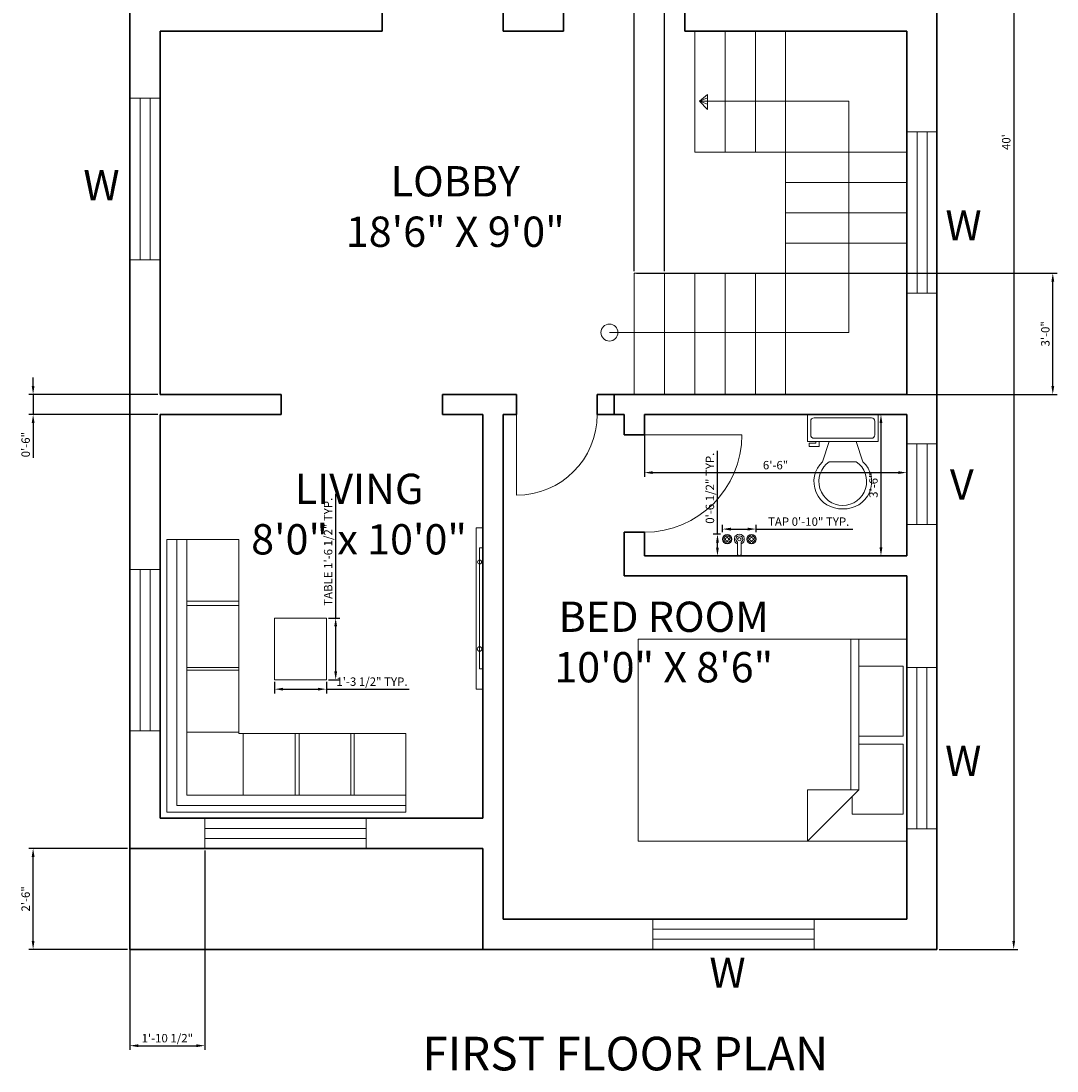
# Model space of a CAD drawing. Units: inches. Extents: x 1827 to 2455, y 1682 to 2281.
# Tile 2 of 3: x 2147 to 2455, y 1682 to 1994. Entities that reach past the tile are written whole.
import ezdxf

# ---------------------------------------------------------------- set-up
doc = ezdxf.new("R2010")
doc.units = ezdxf.units.IN
for name, color, linetype, lineweight in [('A-ANNO-DIMS', 2, 'Continuous', 18), ('A-ANNO-TEXT', 7, 'Continuous', 18), ('A-AREA-IDEN', 7, 'Continuous', 18), ('A-DOOR', 3, 'Continuous', 18), ('A-EQPM', 9, 'Continuous', 18), ('A-FLOR-FIXT', 9, 'Continuous', 18), ('A-FLOR-STRS', 7, 'Continuous', 20), ('A-FURN', 8, 'Continuous', 18), ('A-GLAZ', 4, 'Continuous', 18), ('A-WALL', 7, 'Continuous', 35)]:
    doc.layers.add(name, color=color, linetype=linetype, lineweight=lineweight)
doc.styles.get("Standard").update_dxf_attribs({"font": 'arial.ttf'})
doc.dimstyles.new('ISO-25', dxfattribs={"dimtxt": 2.5, "dimasz": 2.5, "dimexe": 1.25, "dimexo": 0.625, "dimtad": 1, "dimdec": 0, "dimlunit": 3, "dimtxsty": 'Standard', "dimcen": 2.5, "dimadec": 0, "dimazin": 0, "dimtfac": 1, "dimtdec": 0, "dimtmove": 0, "dimatfit": 3, "dimfxl": 1, "dimarcsym": 0})

# ---------------------------------------------------------------- blocks, each defined once
blk = doc.blocks.new('Faucet - Bathroom top')
for p, q in [((-4.107, 0.125), (-4.375, 0.125)), ((-3.75, 0.4788), (-3.75, 0.75)), ((-3.5, 0.482), (-3.5, 0.75)), ((-3.1461, 0.125), (-2.875, 0.125)), ((3.143, 0.125), (2.875, 0.125)), ((3.5, 0.4788), (3.5, 0.75)), ((3.75, 0.482), (3.75, 0.75)), ((4.1039, 0.125), (4.375, 0.125)), ((-4.1039, -0.125), (-4.375, -0.125)), ((-3.75, -0.4821), (-3.75, -0.75)), ((-3.5, -0.4789), (-3.5, -0.75)), ((-3.143, -0.125), (-2.875, -0.125)), ((-0.5, -0.8639), (-0.5, -4.5)), ((0.5, -4.5), (0.5, -0.8631)), ((3.1461, -0.125), (2.875, -0.125)), ((3.5, -0.4821), (3.5, -0.75)), ((3.75, -0.4789), (3.75, -0.75)), ((4.107, -0.125), (4.375, -0.125))]:
    blk.add_line(p, q)
for centre, radius in [((-3.625, 0), 1.375), ((-4.625, 0), 0.2795), ((-3.625, 0), 0.5), ((-3.625, 1), 0.2795), ((-2.625, 0), 0.2795), ((0, 0), 0.5), ((3.625, 0), 1.375), ((2.625, 0), 0.2795), ((3.625, 0), 0.5), ((3.625, 1), 0.2795), ((4.625, 0), 0.2795), ((-3.625, -1), 0.2795), ((3.625, -1), 0.2795)]:
    blk.add_circle(centre, radius)
for centre, radius, start, end in [((-3.625, 0), 1, 105.2407, 164.2093), ((-3.625, 0), 1, 16.44125, 74.07887), ((0, 0), 1.5, 289.6514, 250.3603), ((0, 0), 1, 300.3431, 239.7554), ((3.625, 0), 1, 106.12, 164.0884), ((3.625, 0), 1, 16.23422, 73.90469), ((-3.625, 0), 1, 196.2342, 253.9047), ((-3.625, 0), 1, 286.12, 344.0884), ((3.625, 0), 1, 196.4413, 254.0789), ((3.625, 0), 1, 285.2407, 344.2093), ((0, -4.5), 0.5, 180, 0)]:
    blk.add_arc(centre, radius, start, end)
blk = doc.blocks.new('*U14')
for p, q in [((9.5, -6), (9.5, -2)), ((-10, -8.5), (-8, -8.5)), ((-10, -9.5), (-10, -8.5)), ((-8, -8.5), (-8, -8)), ((-7, -8), (-7, -9.5)), ((-4, -8), (-6, -14)), ((4, -8), (6, -14)), ((-7, -9.5), (-10, -9.5)), ((4, -14), (-4, -14))]:
    blk.add_line(p, q)
blk.add_lwpolyline([(10.5, -8), (10.5, 0), (-10.5, 0), (-10.5, -8)], close=True)
for points in [[(-9.5, -2), (-9.5, -6)], [(8.5, -1), (-8.5, -1)], [(-8.5, -7), (8.5, -7)]]:
    blk.add_lwpolyline(points)
for centre, radius, start, end in [((-8.625, -1.875), 0.8839, 81.8699, 188.1301), ((8.625, -1.875), 0.8839, 351.8699, 98.1301), ((-8.625, -6.125), 0.8839, 171.869898, 278.1301), ((8.625, -6.125), 0.8839, 261.8699, 8.1301), ((-0.4772, -19.9188), 8.0953, 133.01722, 273.38), ((0.0374, -19.8731), 7.127, 124.50543, 269.7), ((-0.0373, -19.8731), 7.127, 270.3, 55.4946), ((0.4773, -19.9188), 8.0953, 266.62, 46.9828)]:
    blk.add_arc(centre, radius, start, end)
blk = doc.blocks.new('Bed - Queen')
for p, q in [((0, -80.00003), (0, 0)), ((0, 0), (59.99999, 0)), ((59.99999, 0), (59.99999, -80.00003)), ((7.99999, -1.2), (28.79998, -1.2)), ((7.99999, -14.4), (7.99999, -1.2)), ((28.79998, -1.2), (28.79998, -14.4)), ((31.19999, -1.2), (51.99999, -1.2)), ((31.19999, -14.4), (31.19999, -1.2)), ((51.99999, -1.2), (51.99999, -16.4)), ((0, -14.4), (44.8, -14.4)), ((59.99999, -29.6), (44.8, -14.4)), ((44.8, -14.4), (44.8, -29.6)), ((44.8, -16.8), (0, -16.8)), ((51.99999, -16.4), (46.79936, -16.4)), ((44.8, -29.6), (59.99999, -29.6)), ((59.99999, -80.00003), (0, -80.00003))]:
    blk.add_line(p, q)
blk = doc.blocks.new('*D16')
at = {"layer": 'A-ANNO-DIMS', "color": 0, "lineweight": -2, "transparency": 16777216}
for p, q in [((2419.98, 2197.92), (2443.42, 2197.92)), ((2442.17, 2195.42), (2442.17, 1720.42)), ((2419.98, 1717.92), (2443.42, 1717.92))]:
    blk.add_line(p, q, dxfattribs=at)
at = {"layer": 'A-ANNO-DIMS', "color": 0, "transparency": 16777216}
for points in [[(2441.75, 2195.42), (2442.59, 2195.42), (2442.17, 2197.92)], [(2441.75, 1720.42), (2442.59, 1720.42), (2442.17, 1717.92)]]:
    blk.add_solid(points, dxfattribs=at)
at = {"layer": 'Defpoints', "color": 0, "transparency": 16777216}
for p in [(2419.36, 2197.92), (2419.36, 1717.92), (2442.17, 1717.92)]:
    blk.add_point(p, dxfattribs=at)
at = {"layer": 'A-ANNO-DIMS', "color": 0, "transparency": 16777216, "insert": (2440.27, 1957.92), "char_height": 2.5, "attachment_point": 5, "rotation": 90}
blk.add_mtext("40'", dxfattribs=at)
blk = doc.blocks.new('*D17')
at = {"layer": 'A-ANNO-DIMS', "color": 0, "lineweight": -2, "transparency": 16777216}
for p, q in [((2332.36, 1876.3), (2332.36, 1858.4)), ((2410.36, 1876.3), (2410.36, 1858.4)), ((2334.86, 1859.65), (2407.86, 1859.65))]:
    blk.add_line(p, q, dxfattribs=at)
at = {"layer": 'A-ANNO-DIMS', "color": 0, "transparency": 16777216}
for points in [[(2334.86, 1860.07), (2334.86, 1859.24), (2332.36, 1859.65)], [(2407.86, 1860.07), (2407.86, 1859.24), (2410.36, 1859.65)]]:
    blk.add_solid(points, dxfattribs=at)
at = {"layer": 'Defpoints', "color": 0, "transparency": 16777216}
for p in [(2332.36, 1876.92), (2410.36, 1876.92), (2410.36, 1859.65)]:
    blk.add_point(p, dxfattribs=at)
at = {"layer": 'A-ANNO-DIMS', "color": 0, "transparency": 16777216, "insert": (2371.36, 1861.55), "char_height": 2.5, "attachment_point": 5}
blk.add_mtext('6\'-6"', dxfattribs=at)
blk = doc.blocks.new('*D18')
at = {"layer": 'A-ANNO-DIMS', "color": 0, "lineweight": -2, "transparency": 16777216}
for p, q in [((2409.73, 1876.92), (2401.45, 1876.92)), ((2402.7, 1874.42), (2402.7, 1837.42)), ((2409.73, 1834.92), (2401.45, 1834.92))]:
    blk.add_line(p, q, dxfattribs=at)
at = {"layer": 'A-ANNO-DIMS', "color": 0, "transparency": 16777216}
for points in [[(2402.29, 1874.42), (2403.12, 1874.42), (2402.7, 1876.92)], [(2402.29, 1837.42), (2403.12, 1837.42), (2402.7, 1834.92)]]:
    blk.add_solid(points, dxfattribs=at)
at = {"layer": 'Defpoints', "color": 0, "transparency": 16777216}
for p in [(2410.36, 1876.92), (2402.7, 1834.92), (2410.36, 1834.92)]:
    blk.add_point(p, dxfattribs=at)
at = {"layer": 'A-ANNO-DIMS', "color": 0, "transparency": 16777216, "insert": (2400.8, 1855.92), "char_height": 2.5, "attachment_point": 5, "rotation": 90}
blk.add_mtext('3\'-6"', dxfattribs=at)
blk = doc.blocks.new('WIN-48IN')
for p, q in [((48, 9), (0, 9)), ((0, 9), (0, 0)), ((48, 0), (48, 9)), ((48, 6), (0, 6)), ((0, 3), (48, 3)), ((0, 0), (48, 0))]:
    blk.add_line(p, q)
blk = doc.blocks.new('VENT-24IN')
for p, q in [((0, 24), (0, 0)), ((0, 24), (9, 24)), ((3, 24), (3, 0)), ((6, 0), (6, 24)), ((9, 0), (9, 24)), ((0, 0), (9, 0))]:
    blk.add_line(p, q)
blk = doc.blocks.new('DOOR-29IN-SINGLE')
blk.add_line((0, 0), (0, 29))
blk.add_arc((0, 0), 29, 0, 90)
blk = doc.blocks.new('SOFA-L-SECTIONAL')
for p, q in [((0, 81.06), (0, 23.78)), ((3, 81.06), (3, 23.78)), ((6, 81.06), (6, 23.78)), ((21.43, 81.06), (21.43, 23.78)), ((0, 23.78), (0, 5)), ((3, 23.78), (3, 5)), ((6, 23.78), (6, 5)), ((21.43, 23.38), (21.43, 23.78)), ((21.43, 23.78), (21.43, 23.38)), ((22.69, 23.38), (21.43, 23.38)), ((21.43, 23.38), (39.33, 23.38)), ((22.69, 5), (22.69, 23.38)), ((39.33, 23.38), (71.09, 23.38)), ((0, 5), (0, 0)), ((3, 5), (3, 2)), ((22.69, 5), (6, 5)), ((71.09, 5), (22.69, 5)), ((71.09, 5), (71.09, 0)), ((6, 2), (3, 2)), ((22.69, 2), (6, 2)), ((71.09, 2), (22.69, 2)), ((6, 0), (0, 0)), ((22.69, 0), (6, 0)), ((71.09, 0), (22.69, 0))]:
    blk.add_line(p, q)
for points in [[(6, 81.06), (21.43, 81.06), (21.43, 62.67), (6, 62.67)], [(6, 61.41), (21.43, 61.41), (21.43, 43.03), (6, 43.03)], [(6, 42.16), (21.43, 42.16), (21.43, 23.78), (6, 23.78)], [(22.69, 23.38), (38.12, 23.38), (38.12, 5), (22.69, 5)], [(39.33, 23.38), (54.76, 23.38), (54.76, 5), (39.33, 5)], [(55.66, 23.38), (71.09, 23.38), (71.09, 5), (55.66, 5)]]:
    blk.add_lwpolyline(points, close=True)
blk = doc.blocks.new('TABLE-OCCASIONAL')
blk.add_lwpolyline([(0, 18.39), (15.43, 18.39), (15.43, 0), (0, 0)], close=True)
blk = doc.blocks.new('*D33')
at = {"layer": 'A-ANNO-DIMS', "color": 0, "lineweight": -2, "transparency": 16777216}
for p, q in [((2355.59, 1841.99), (2355.59, 1844.11)), ((2358.09, 1842.86), (2363.09, 1842.86)), ((2365.59, 1841.99), (2365.59, 1844.11)), ((2365.59, 1842.86), (2394.34, 1842.86))]:
    blk.add_line(p, q, dxfattribs=at)
at = {"layer": 'A-ANNO-DIMS', "color": 0, "transparency": 16777216}
for points in [[(2358.09, 1843.28), (2358.09, 1842.44), (2355.59, 1842.86)], [(2363.09, 1843.28), (2363.09, 1842.44), (2365.59, 1842.86)]]:
    blk.add_solid(points, dxfattribs=at)
at = {"layer": 'Defpoints', "color": 0, "transparency": 16777216}
for p in [(2365.59, 1842.86), (2355.59, 1841.36), (2365.59, 1841.36)]:
    blk.add_point(p, dxfattribs=at)
at = {"layer": 'A-ANNO-DIMS', "color": 0, "transparency": 16777216, "insert": (2381.21, 1844.76), "char_height": 2.5, "attachment_point": 5}
blk.add_mtext('TAP 0\'-10" TYP.', dxfattribs=at)
blk = doc.blocks.new('*D34')
at = {"layer": 'A-ANNO-DIMS', "color": 0, "lineweight": -2, "transparency": 16777216}
for p, q in [((2354.09, 1841.36), (2354.09, 1866.17)), ((2354.96, 1841.36), (2352.84, 1841.36)), ((2354.09, 1837.36), (2354.09, 1838.86)), ((2354.96, 1834.86), (2352.84, 1834.86))]:
    blk.add_line(p, q, dxfattribs=at)
at = {"layer": 'A-ANNO-DIMS', "color": 0, "transparency": 16777216}
for points in [[(2353.67, 1838.86), (2354.5, 1838.86), (2354.09, 1841.36)], [(2353.67, 1837.36), (2354.5, 1837.36), (2354.09, 1834.86)]]:
    blk.add_solid(points, dxfattribs=at)
at = {"layer": 'Defpoints', "color": 0, "transparency": 16777216}
for p in [(2354.09, 1841.36), (2355.59, 1841.36), (2355.59, 1834.86)]:
    blk.add_point(p, dxfattribs=at)
at = {"layer": 'A-ANNO-DIMS', "color": 0, "transparency": 16777216, "insert": (2352.17, 1855.02), "char_height": 2.5, "attachment_point": 5, "rotation": 90}
blk.add_mtext('0\'-6 1/2" TYP.', dxfattribs=at)
blk = doc.blocks.new('*D47')
at = {"layer": 'A-ANNO-DIMS', "color": 0, "lineweight": -2, "transparency": 16777216}
for p, q in [((2240.58, 1816.42), (2240.58, 1853.33)), ((2238.45, 1816.42), (2241.83, 1816.42)), ((2240.58, 1800.53), (2240.58, 1813.92)), ((2238.45, 1798.03), (2241.83, 1798.03))]:
    blk.add_line(p, q, dxfattribs=at)
at = {"layer": 'A-ANNO-DIMS', "color": 0, "transparency": 16777216}
for points in [[(2240.16, 1813.92), (2241, 1813.92), (2240.58, 1816.42)], [(2240.16, 1800.53), (2241, 1800.53), (2240.58, 1798.03)]]:
    blk.add_solid(points, dxfattribs=at)
at = {"layer": 'Defpoints', "color": 0, "transparency": 16777216}
for p in [(2237.82, 1816.42), (2240.58, 1816.42), (2237.82, 1798.03)]:
    blk.add_point(p, dxfattribs=at)
at = {"layer": 'A-ANNO-DIMS', "color": 0, "transparency": 16777216, "insert": (2238.66, 1836.12), "char_height": 2.5, "attachment_point": 5, "rotation": 90}
blk.add_mtext('TABLE 1\'-6 1/2" TYP.', dxfattribs=at)
blk = doc.blocks.new('*D48')
at = {"layer": 'A-ANNO-DIMS', "color": 0, "lineweight": -2, "transparency": 16777216}
for p, q in [((2222.4, 1797.41), (2222.4, 1794.02)), ((2224.9, 1795.27), (2235.32, 1795.27)), ((2237.82, 1797.41), (2237.82, 1794.02)), ((2237.82, 1795.27), (2262.4, 1795.27))]:
    blk.add_line(p, q, dxfattribs=at)
at = {"layer": 'A-ANNO-DIMS', "color": 0, "transparency": 16777216}
for points in [[(2224.9, 1795.69), (2224.9, 1794.86), (2222.4, 1795.27)], [(2235.32, 1795.69), (2235.32, 1794.86), (2237.82, 1795.27)]]:
    blk.add_solid(points, dxfattribs=at)
at = {"layer": 'Defpoints', "color": 0, "transparency": 16777216}
for p in [(2222.4, 1798.03), (2237.82, 1798.03), (2237.82, 1795.27)]:
    blk.add_point(p, dxfattribs=at)
at = {"layer": 'A-ANNO-DIMS', "color": 0, "transparency": 16777216, "insert": (2251.36, 1797.19), "char_height": 2.5, "attachment_point": 5}
blk.add_mtext('1\'-3 1/2" TYP.', dxfattribs=at)
blk = doc.blocks.new('*D55')
at = {"layer": 'A-ANNO-DIMS', "color": 0, "lineweight": -2, "transparency": 16777216}
for p, q in [((2329.98, 1918.92), (2455.04, 1918.92)), ((2453.79, 1885.42), (2453.79, 1916.42)), ((2329.98, 1882.92), (2455.04, 1882.92))]:
    blk.add_line(p, q, dxfattribs=at)
at = {"layer": 'A-ANNO-DIMS', "color": 0, "transparency": 16777216}
for points in [[(2453.37, 1916.42), (2454.21, 1916.42), (2453.79, 1918.92)], [(2453.37, 1885.42), (2454.21, 1885.42), (2453.79, 1882.92)]]:
    blk.add_solid(points, dxfattribs=at)
at = {"layer": 'Defpoints', "color": 0, "transparency": 16777216}
for p in [(2329.36, 1918.92), (2453.79, 1918.92), (2329.36, 1882.92)]:
    blk.add_point(p, dxfattribs=at)
at = {"layer": 'A-ANNO-DIMS', "color": 0, "transparency": 16777216, "insert": (2451.89, 1900.92), "char_height": 2.5, "attachment_point": 5, "rotation": 90}
blk.add_mtext('3\'-0"', dxfattribs=at)
blk = doc.blocks.new('*D56')
at = {"layer": 'A-ANNO-DIMS', "color": 0, "lineweight": -2, "transparency": 16777216}
for p, q in [((2329.36, 1919.55), (2329.36, 2278.82)), ((2331.86, 2277.57), (2335.86, 2277.57)), ((2338.36, 1919.55), (2338.36, 2278.82))]:
    blk.add_line(p, q, dxfattribs=at)
at = {"layer": 'A-ANNO-DIMS', "color": 0, "transparency": 16777216}
for points in [[(2331.86, 2277.99), (2331.86, 2277.16), (2329.36, 2277.57)], [(2335.86, 2277.99), (2335.86, 2277.16), (2338.36, 2277.57)]]:
    blk.add_solid(points, dxfattribs=at)
at = {"layer": 'Defpoints', "color": 0, "transparency": 16777216}
for p in [(2338.36, 2277.57), (2329.36, 1918.92), (2338.36, 1918.92)]:
    blk.add_point(p, dxfattribs=at)
at = {"layer": 'A-ANNO-DIMS', "color": 0, "transparency": 16777216, "insert": (2333.86, 2279.47), "char_height": 2.5, "attachment_point": 5}
blk.add_mtext('0\'-9"', dxfattribs=at)
blk = doc.blocks.new('*D58')
at = {"layer": 'A-ANNO-DIMS', "color": 0, "lineweight": -2, "transparency": 16777216}
for p, q in [((2178.73, 1747.92), (2149.37, 1747.92)), ((2150.62, 1720.42), (2150.62, 1745.42)), ((2178.73, 1717.92), (2149.37, 1717.92))]:
    blk.add_line(p, q, dxfattribs=at)
at = {"layer": 'A-ANNO-DIMS', "color": 0, "transparency": 16777216}
for points in [[(2150.2, 1745.42), (2151.04, 1745.42), (2150.62, 1747.92)], [(2150.2, 1720.42), (2151.04, 1720.42), (2150.62, 1717.92)]]:
    blk.add_solid(points, dxfattribs=at)
at = {"layer": 'Defpoints', "color": 0, "transparency": 16777216}
for p in [(2150.62, 1747.92), (2179.36, 1747.92), (2179.36, 1717.92)]:
    blk.add_point(p, dxfattribs=at)
at = {"layer": 'A-ANNO-DIMS', "color": 0, "transparency": 16777216, "insert": (2148.72, 1732.92), "char_height": 2.5, "attachment_point": 5, "rotation": 90}
blk.add_mtext('2\'-6"', dxfattribs=at)
blk = doc.blocks.new('*D60')
at = {"layer": 'A-ANNO-DIMS', "color": 0, "lineweight": -2, "transparency": 16777216}
for p, q in [((2179.36, 1747.3), (2179.36, 1688.02)), ((2201.68, 1747.26), (2201.68, 1688.02)), ((2181.86, 1689.27), (2199.18, 1689.27))]:
    blk.add_line(p, q, dxfattribs=at)
at = {"layer": 'A-ANNO-DIMS', "color": 0, "transparency": 16777216}
for points in [[(2181.86, 1689.69), (2181.86, 1688.86), (2179.36, 1689.27)], [(2199.18, 1689.69), (2199.18, 1688.86), (2201.68, 1689.27)]]:
    blk.add_solid(points, dxfattribs=at)
at = {"layer": 'Defpoints', "color": 0, "transparency": 16777216}
for p in [(2179.36, 1747.92), (2201.68, 1747.88), (2201.68, 1689.27)]:
    blk.add_point(p, dxfattribs=at)
at = {"layer": 'A-ANNO-DIMS', "color": 0, "transparency": 16777216, "insert": (2190.52, 1691.19), "char_height": 2.5, "attachment_point": 5}
blk.add_mtext('1\'-10 1/2"', dxfattribs=at)
blk = doc.blocks.new('*D61')
at = {"layer": 'A-ANNO-DIMS', "color": 0, "lineweight": -2, "transparency": 16777216}
for p, q in [((2150.62, 1885.42), (2150.62, 1887.92)), ((2187.73, 1882.92), (2149.37, 1882.92)), ((2150.62, 1882.92), (2150.62, 1876.92)), ((2187.73, 1876.92), (2149.37, 1876.92)), ((2150.62, 1874.42), (2150.62, 1864.03))]:
    blk.add_line(p, q, dxfattribs=at)
at = {"layer": 'A-ANNO-DIMS', "color": 0, "transparency": 16777216}
for points in [[(2150.2, 1885.42), (2151.04, 1885.42), (2150.62, 1882.92)], [(2150.2, 1874.42), (2151.04, 1874.42), (2150.62, 1876.92)]]:
    blk.add_solid(points, dxfattribs=at)
at = {"layer": 'Defpoints', "color": 0, "transparency": 16777216}
for p in [(2188.36, 1882.92), (2150.62, 1876.92), (2188.36, 1876.92)]:
    blk.add_point(p, dxfattribs=at)
at = {"layer": 'A-ANNO-DIMS', "color": 0, "transparency": 16777216, "insert": (2148.72, 1867.97), "char_height": 2.5, "attachment_point": 5, "rotation": 90}
blk.add_mtext('0\'-6"', dxfattribs=at)

msp = doc.modelspace()

# ---------------------------------------------------------------- linework, layer by layer
at = {"layer": 'A-DOOR'}
msp.add_line((2294.36, 1876.92), (2294.36, 1852.92), dxfattribs=at)
msp.add_arc((2294.36, 1876.92), 24, 270, 0, dxfattribs=at)
at = {"layer": 'A-EQPM'}
for p, q in [((2282.36, 1795.27), (2282.36, 1843.27)), ((2282.36, 1843.27), (2284.36, 1843.27)), ((2284.36, 1843.27), (2284.36, 1795.27)), ((2284.36, 1843.27), (2284.36, 1837.27)), ((2284.36, 1837.27), (2283.36, 1837.27)), ((2283.36, 1837.27), (2283.36, 1801.27)), ((2283.36, 1801.27), (2284.36, 1801.27)), ((2284.36, 1795.27), (2282.36, 1795.27))]:
    msp.add_line(p, q, dxfattribs=at)
for centre, radius in [((2283.36, 1833.07), 0.594), ((2283.36, 1807.22), 0.691)]:
    msp.add_circle(centre, radius, dxfattribs=at)
at = {"layer": 'A-FLOR-STRS'}
for p, q in [((2347.36, 1954.92), (2347.36, 1990.92)), ((2356.36, 1954.92), (2356.36, 1990.92)), ((2365.36, 1954.92), (2365.36, 1990.92)), ((2374.36, 1882.92), (2374.36, 1990.92)), ((2348.79, 1970.13), (2351.1, 1972.07)), ((2348.79, 1970.13), (2351.1, 1971.06)), ((2351.1, 1967.6), (2348.79, 1970.13)), ((2351.1, 1970.04), (2348.79, 1970.13)), ((2351.1, 1969.2), (2348.79, 1970.13)), ((2351.1, 1970.04), (2351.1, 1972.07)), ((2351.1, 1972.07), (2351.1, 1967.6)), ((2351.1, 1971.06), (2351.1, 1969.2)), ((2393.19, 1970.04), (2351.1, 1970.04)), ((2393.19, 1901.29), (2393.19, 1970.04)), ((2410.36, 1954.92), (2347.36, 1954.92)), ((2410.36, 1945.92), (2374.36, 1945.92)), ((2410.36, 1936.92), (2374.36, 1936.92)), ((2410.36, 1927.92), (2374.36, 1927.92)), ((2410.36, 1918.92), (2329.36, 1918.92)), ((2329.36, 1882.92), (2329.36, 1918.92)), ((2338.36, 1882.92), (2338.36, 1918.92)), ((2347.36, 1882.92), (2347.36, 1918.92)), ((2356.36, 1882.92), (2356.36, 1918.92)), ((2365.36, 1882.92), (2365.36, 1918.92)), ((2321.96, 1901.29), (2393.19, 1901.29))]:
    msp.add_line(p, q, dxfattribs=at)
msp.add_circle((2321.96, 1901.29), 2.53, dxfattribs=at)
at = {"layer": 'A-FURN'}
msp.add_line((2196.37, 1839.78), (2190.37, 1839.78), dxfattribs=at)
at = {"layer": 'A-WALL'}
for p, q in [((2179.36, 2197.92), (2179.36, 1717.92)), ((2419.36, 1717.92), (2419.36, 2197.92)), ((2254.36, 1990.92), (2254.36, 1996.92)), ((2290.36, 1996.92), (2290.36, 1990.92)), ((2308.36, 1996.92), (2308.36, 1990.92)), ((2344.36, 1990.92), (2344.36, 1996.92)), ((2188.36, 1990.92), (2188.36, 1882.92)), ((2254.36, 1990.92), (2188.36, 1990.92)), ((2308.36, 1990.92), (2290.36, 1990.92)), ((2410.36, 1990.92), (2344.36, 1990.92)), ((2410.36, 1882.92), (2410.36, 1990.92)), ((2224.36, 1882.92), (2188.36, 1882.92)), ((2224.36, 1882.92), (2224.36, 1876.92)), ((2272.36, 1876.92), (2272.36, 1882.92)), ((2294.36, 1882.92), (2272.36, 1882.92)), ((2294.36, 1876.92), (2294.36, 1882.92)), ((2318.36, 1882.92), (2323.36, 1882.92)), ((2318.36, 1882.92), (2318.36, 1876.92)), ((2410.36, 1882.92), (2323.36, 1882.92)), ((2323.36, 1882.92), (2323.36, 1876.92)), ((2188.36, 1876.92), (2188.36, 1756.92)), ((2224.36, 1876.92), (2188.36, 1876.92)), ((2284.36, 1876.92), (2272.36, 1876.92)), ((2284.36, 1876.92), (2272.36, 1876.92)), ((2284.36, 1756.92), (2284.36, 1876.92)), ((2294.36, 1876.92), (2290.36, 1876.92)), ((2290.36, 1726.92), (2290.36, 1876.92)), ((2290.36, 1876.92), (2294.36, 1876.92)), ((2326.36, 1876.92), (2318.36, 1876.92)), ((2326.36, 1876.92), (2326.36, 1870.92)), ((2326.36, 1870.92), (2326.36, 1876.92)), ((2410.36, 1876.92), (2332.36, 1876.92)), ((2332.36, 1870.92), (2332.36, 1876.92)), ((2410.36, 1834.92), (2410.36, 1876.92)), ((2326.36, 1870.92), (2332.36, 1870.92)), ((2326.36, 1870.92), (2332.36, 1870.92)), ((2326.36, 1828.92), (2326.36, 1841.92)), ((2332.36, 1841.92), (2326.36, 1841.92)), ((2332.36, 1834.92), (2332.36, 1841.92)), ((2410.36, 1834.92), (2332.36, 1834.92)), ((2410.36, 1828.92), (2326.36, 1828.92)), ((2410.36, 1726.92), (2410.36, 1828.92)), ((2284.36, 1756.92), (2188.36, 1756.92)), ((2188.36, 1747.92), (2179.36, 1747.92)), ((2284.36, 1747.92), (2188.36, 1747.92)), ((2284.36, 1717.92), (2284.36, 1747.92)), ((2290.36, 1726.92), (2410.36, 1726.92)), ((2179.36, 1717.92), (2419.36, 1717.92))]:
    msp.add_line(p, q, dxfattribs=at)

# ---------------------------------------------------------------- block references
at = {"layer": 'A-DOOR', "rotation": 270.0000000000005}
msp.add_blockref('DOOR-29IN-SINGLE', (2332.36, 1870.92), dxfattribs=at)
at = {"layer": 'A-FLOR-FIXT'}
for name, p in [('*U14', (2391.34, 1876.9)), ('Faucet - Bathroom top', (2360.59, 1839.86))]:
    msp.add_blockref(name, p, dxfattribs=at)
at = {"layer": 'A-FURN'}
for name, p in [('SOFA-L-SECTIONAL', (2190.37, 1758.72)), ('TABLE-OCCASIONAL', (2222.4, 1798.03))]:
    msp.add_blockref(name, p, dxfattribs=at)
at = {"layer": 'A-FURN', "rotation": 270}
msp.add_blockref('Bed - Queen', (2410.5, 1810.11), dxfattribs=at)
at = {"layer": 'A-GLAZ'}
for name, p, rotation in [('WIN-48IN', (2188.43, 1922.96), 90.00000000000104), ('WIN-48IN', (2419.44, 1912.97), 90.00000000000072), ('VENT-24IN', (2419.4, 1868.26), 180), ('WIN-48IN', (2188.44, 1782.86), 90.00000000000081), ('WIN-48IN', (2419.36, 1753.76), 89.99999999999991)]:
    msp.add_blockref(name, p, dxfattribs=dict(at, rotation=rotation))
for p in [(2201.68, 1747.88), (2334.84, 1717.92)]:
    msp.add_blockref('WIN-48IN', p, dxfattribs=at)

# ---------------------------------------------------------------- texts
at = {"layer": 'A-ANNO-TEXT', "attachment_point": 1}
for s, width, insert, char_height in [('\\pxqc;W', 56.1832, (2142.85, 1949.61), 9), ('\\pxqc;W', 56.1832, (2399.16, 1937.67), 9), ('\\pxqc;V', 51.3012, (2401.08, 1860.62), 9), ('\\pxqc;W', 56.1832, (2399.07, 1778.45), 9), ('\\pxqc;W', 56.1832, (2328.98, 1715.48), 9), ('\\P\\pxqc;FIRST FLOOR PLAN', 180.0587, (2236.64, 1708.6), 10)]:
    msp.add_mtext_dynamic_manual_height_columns(s, width=width, gutter_width=12.5, heights=[0], dxfattribs=dict(at, insert=insert, char_height=char_height))
at = {"layer": 'A-AREA-IDEN', "char_height": 9, "attachment_point": 1}
for s, width, insert in [('\\pxqc;LOBBY \\P18\'6" X 9\'0"', 93.1734, (2229.55, 1950.78)), ('\\pxqc;LIVING\\P8\'0" x 10\'0"', 73.6598, (2210.7, 1859.33)), ('\\pxqc;BED ROOM\\P10\'0" X 8\'6" ', 81.5614, (2297.33, 1821.3))]:
    msp.add_mtext_dynamic_manual_height_columns(s, width=width, gutter_width=12.5, heights=[0], dxfattribs=dict(at, insert=insert))

# ---------------------------------------------------------------- dimensions: what is measured, and where the dimension line sits
at = {"layer": 'A-ANNO-DIMS'}
for base, p1, p2, override, picture, middle in [((2338.36, 2277.57), (2329.36, 1918.92), (2338.36, 1918.92), {"dimdec": 1, "dimlfac": 1, "dimrnd": 0, "dimzin": 1, "dimdsep": 46, "dimlunit": 4, "dimfrac": 2}, '*D56', (2333.86, 2279.47)), ((2410.36, 1859.65), (2332.36, 1876.92), (2410.36, 1876.92), {"dimclrd": 0, "dimclre": 0, "dimclrt": 0}, '*D17', (2371.36, 1861.55)), ((2201.68, 1689.27), (2179.36, 1747.92), (2201.68, 1747.88), {"dimdec": 1, "dimlfac": 1, "dimrnd": 0, "dimzin": 1, "dimdsep": 46, "dimlunit": 4, "dimfrac": 2}, '*D60', (2190.52, 1691.19))]:
    dim = msp.add_linear_dim(base=base, p1=p1, p2=p2, dimstyle='ISO-25', override=override, dxfattribs=at)
    dim.commit()
    dim.dimension.update_dxf_attribs({"geometry": picture, "text_midpoint": middle})
for base, p1, p2, override, picture, middle in [((2442.17, 1717.92), (2419.36, 2197.92), (2419.36, 1717.92), {"dimclrd": 0, "dimclre": 0, "dimclrt": 0}, '*D16', (2440.27, 1957.92)), ((2453.79, 1918.92), (2329.36, 1882.92), (2329.36, 1918.92), {"dimdec": 1, "dimlfac": 1, "dimrnd": 0, "dimzin": 1, "dimdsep": 46, "dimlunit": 4, "dimfrac": 2}, '*D55', (2451.89, 1900.92)), ((2150.62, 1876.92), (2188.36, 1882.92), (2188.36, 1876.92), {"dimdec": 1, "dimlfac": 1, "dimrnd": 0, "dimzin": 1, "dimdsep": 46, "dimlunit": 4, "dimfrac": 2}, '*D61', (2148.72, 1867.97)), ((2402.7, 1834.92), (2410.36, 1876.92), (2410.36, 1834.92), {"dimclrd": 0, "dimclre": 0, "dimclrt": 0}, '*D18', (2400.8, 1855.92)), ((2150.62, 1747.92), (2179.36, 1717.92), (2179.36, 1747.92), {"dimdec": 1, "dimlfac": 1, "dimrnd": 0, "dimzin": 1, "dimdsep": 46, "dimlunit": 4, "dimfrac": 2}, '*D58', (2148.72, 1732.92))]:
    dim = msp.add_linear_dim(base=base, p1=p1, p2=p2, angle=90, dimstyle='ISO-25', override=override, dxfattribs=at)
    dim.commit()
    dim.dimension.update_dxf_attribs({"geometry": picture, "text_midpoint": middle})
for base, p1, p2, text, picture, middle in [((2354.09, 1841.36), (2355.59, 1834.86), (2355.59, 1841.36), '<> TYP.', '*D34', (2352.17, 1855.02)), ((2240.58, 1816.42), (2237.82, 1798.03), (2237.82, 1816.42), 'TABLE <> TYP.', '*D47', (2238.66, 1836.12))]:
    dim = msp.add_linear_dim(base=base, p1=p1, p2=p2, angle=90, text=text, dimstyle='ISO-25', override={"dimdec": 1, "dimlfac": 1, "dimrnd": 0, "dimzin": 1, "dimdsep": 46, "dimlunit": 4, "dimfrac": 2}, dxfattribs=at)
    dim.commit()
    dim.dimension.update_dxf_attribs({"geometry": picture, "text_midpoint": middle})
for base, p1, p2, text, picture, middle in [((2365.59, 1842.86), (2355.59, 1841.36), (2365.59, 1841.36), 'TAP <> TYP.', '*D33', (2381.21, 1844.76)), ((2237.82, 1795.27), (2222.4, 1798.03), (2237.82, 1798.03), '<> TYP.', '*D48', (2251.36, 1797.19))]:
    dim = msp.add_linear_dim(base=base, p1=p1, p2=p2, text=text, dimstyle='ISO-25', override={"dimdec": 1, "dimlfac": 1, "dimrnd": 0, "dimzin": 1, "dimdsep": 46, "dimlunit": 4, "dimfrac": 2}, dxfattribs=at)
    dim.commit()
    dim.dimension.update_dxf_attribs({"geometry": picture, "text_midpoint": middle})

doc.saveas('drawing.dxf')
